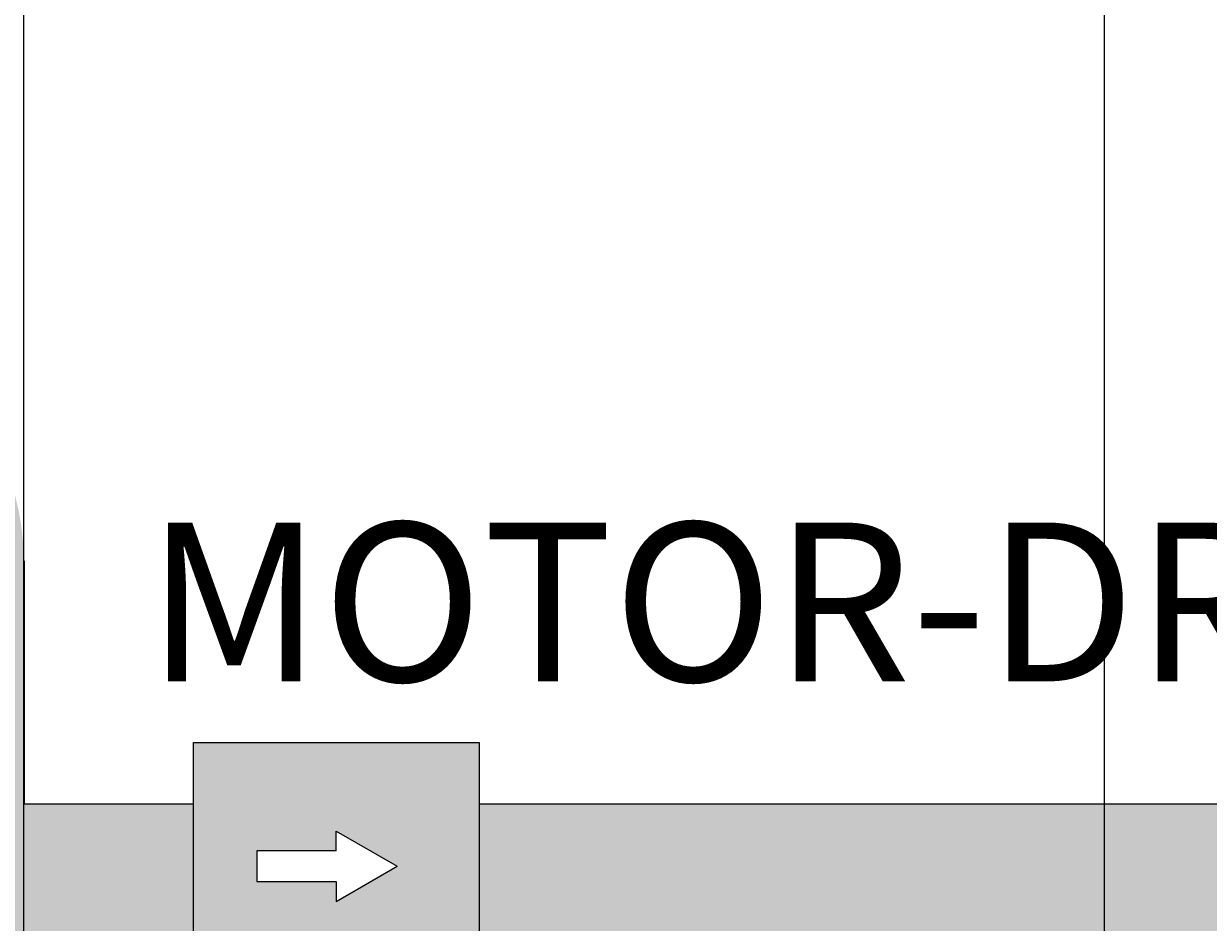
# Model space of a CAD drawing. Units: millimetres. Extents: x -11 to 280, y -4 to 208.
# Tile 41 of 55: x 91 to 121, y 106 to 128. Entities that reach past the tile are written whole.
import ezdxf

# ---------------------------------------------------------------- set-up
doc = ezdxf.new("R2010")
doc.units = ezdxf.units.MM
for name, color, linetype, lineweight in [('M-ANNO-TEXT', 7, 'Continuous', 18), ('M-DIMS', 2, 'Continuous', 18), ('M-HYDR-EQPM', 7, 'Continuous', 35), ('M-HYDR-PRES', 7, 'Continuous', 25), ('M-HYDR-SUCT', 7, 'Continuous', 25), ('M-HYDR-SYMB', 7, 'Continuous', 18), ('M-HYDR-VALV', 7, 'Continuous', 25)]:
    doc.layers.add(name, color=color, linetype=linetype, lineweight=lineweight)
doc.layers.add('M-HYDR-PRES-PATT', color=240, linetype='Continuous', lineweight=13, true_color=0xed1f24)
doc.layers.add('M-HYDR-SUCT-PATT', color=221, linetype='Continuous', lineweight=13, true_color=0xff7fdf)
doc.styles.get("Standard").update_dxf_attribs({"font": 'arial.ttf'})
doc.dimstyles.get("Standard").update_dxf_attribs({"dimtxt": 0.18, "dimasz": 0.18, "dimexe": 0.18, "dimexo": 0.0625, "dimgap": 0.09, "dimtad": 0, "dimtih": 1, "dimtoh": 1, "dimdec": 4, "dimzin": 0, "dimdsep": 46, "dimtxsty": 'Standard', "dimcen": 0.09, "dimadec": 0, "dimazin": 0, "dimtfac": 1, "dimtdec": 4, "dimtofl": 0, "dimtmove": 0, "dimatfit": 3, "dimfxl": 1, "dimtolj": 1, "dimtzin": 0, "dimarcsym": 0})

# ---------------------------------------------------------------- blocks, each defined once
blk = doc.blocks.new('HYDR-FLOW-ARROW')
for p, q in [((2, 1.272), (2, 1.772)), ((2, 1.772), (3.535, 0.886)), ((2, 1.272), (0, 1.272)), ((0, 1.272), (0, 0.5)), ((2, 0), (3.535, 0.886)), ((0, 0.5), (2, 0.5)), ((2, 0.5), (2, 0))]:
    blk.add_line(p, q)
blk = doc.blocks.new('*D5')
at = {"layer": 'Defpoints', "color": 0, "transparency": 16777216}
for p in [(24.759, 192.645), (-10.087, 11.435), (261.686, 11.435)]:
    blk.add_point(p, dxfattribs=at)
at = {"layer": 'M-DIMS', "color": 0, "lineweight": -2, "transparency": 16777216}
for p, q in [((24.696, 192.645), (-10.267, 192.645)), ((-10.087, 192.465), (-10.087, 102.222)), ((-10.087, 11.615), (-10.087, 101.858)), ((261.624, 11.435), (-10.267, 11.435))]:
    blk.add_line(p, q, dxfattribs=at)
at = {"layer": 'M-DIMS', "color": 0, "transparency": 16777216}
for points in [[(-10.117, 192.465), (-10.057, 192.465), (-10.087, 192.645)], [(-10.117, 11.615), (-10.057, 11.615), (-10.087, 11.435)]]:
    blk.add_solid(points, dxfattribs=at)
at = {"layer": 'M-DIMS', "color": 0, "transparency": 16777216, "insert": (-10.087, 102.04), "char_height": 0.18, "attachment_point": 5}
blk.add_mtext('\\A1;181.2', dxfattribs=at)
blk = doc.blocks.new('*D11')
at = {"layer": 'Defpoints', "color": 0, "transparency": 16777216}
for p in [(118.514, 207.495), (91.3, 98.149), (118.514, 96.485)]:
    blk.add_point(p, dxfattribs=at)
at = {"layer": 'M-DIMS', "color": 0, "lineweight": -2, "transparency": 16777216}
for p, q in [((91.3, 98.212), (91.3, 207.675)), ((118.514, 96.547), (118.514, 207.675)), ((91.48, 207.495), (104.442, 207.495)), ((118.334, 207.495), (105.372, 207.495))]:
    blk.add_line(p, q, dxfattribs=at)
at = {"layer": 'M-DIMS', "color": 0, "transparency": 16777216}
for points in [[(91.48, 207.525), (91.48, 207.465), (91.3, 207.495)], [(118.334, 207.525), (118.334, 207.465), (118.514, 207.495)]]:
    blk.add_solid(points, dxfattribs=at)
at = {"layer": 'M-DIMS', "color": 0, "transparency": 16777216, "insert": (104.907, 207.495), "char_height": 0.18, "attachment_point": 5}
blk.add_mtext('\\A1;27.214', dxfattribs=at)
blk = doc.blocks.new('*D12')
at = {"layer": 'Defpoints', "color": 0, "transparency": 16777216}
for p in [(173.804, 207.495), (118.514, 96.485), (173.804, 89.387)]:
    blk.add_point(p, dxfattribs=at)
at = {"layer": 'M-DIMS', "color": 0, "lineweight": -2, "transparency": 16777216}
for p, q in [((118.514, 96.547), (118.514, 207.675)), ((173.804, 89.45), (173.804, 207.675)), ((118.694, 207.495), (145.765, 207.495)), ((173.624, 207.495), (146.553, 207.495))]:
    blk.add_line(p, q, dxfattribs=at)
at = {"layer": 'M-DIMS', "color": 0, "transparency": 16777216}
for points in [[(118.694, 207.525), (118.694, 207.465), (118.514, 207.495)], [(173.624, 207.525), (173.624, 207.465), (173.804, 207.495)]]:
    blk.add_solid(points, dxfattribs=at)
at = {"layer": 'M-DIMS', "color": 0, "transparency": 16777216, "insert": (146.159, 207.495), "char_height": 0.18, "attachment_point": 5}
blk.add_mtext('\\A1;55.29', dxfattribs=at)

msp = doc.modelspace()

# ---------------------------------------------------------------- hatches: boundary and pattern name
at = {"layer": 'M-HYDR-PRES-PATT'}
h = msp.add_hatch(color=256, dxfattribs=at)
h.set_gradient(color1=(237, 31, 36), color2=(237, 31, 36), tint=1)
h.paths.add_polyline_path([(232.2, 133.1228), (228.7, 133.1228), (228.7, 108.8141), (102.7646, 108.8141), (102.7646, 105.3141), (232.2, 105.3141)])
h.paths.add_polyline_path([(128.8433, 105.3141), (125.3433, 105.3141), (125.3433, 91.7099, 1), (128.8433, 91.7099)])
h.paths.add_polyline_path([(229.1617, 78.7098), (196.7745, 78.7098, -0.4142136), (191.7745, 83.7098), (191.7745, 105.3141), (188.2745, 105.3141), (188.2745, 80.2098, 0.4142136), (193.2745, 75.2098), (225.6617, 75.2098), (225.6617, 43.5991), (229.1617, 43.5991)])
h.paths.add_polyline_path([(102.7646, 110.3704), (95.5776, 110.3704), (95.5776, 103.9022), (102.7646, 103.9022)])
h.paths.add_polyline_path([(100.7059, 107.2502), (99.1711, 106.3641), (99.1711, 106.8641), (97.1711, 106.8641), (97.1711, 107.6363), (99.1711, 107.6363), (99.1711, 108.1363)], flags=16)
h.paths.add_polyline_path([(234.6119, 138.4081), (226.5106, 138.4081), (226.5106, 133.1228), (234.6119, 133.1228)])
h.paths.add_polyline_path([(231.1963, 135.7055), (230.2965, 134.1786), (229.4241, 135.7213), (229.9241, 135.7168), (229.9418, 137.7167), (230.7141, 137.7099), (230.6963, 135.71)], flags=16)
at = {"layer": 'M-HYDR-SUCT-PATT'}
h = msp.add_hatch(color=256, dxfattribs=at)
h.set_gradient(color1=(255, 127, 223), color2=(255, 127, 223), tint=1, name='INVCYLINDER')
h.paths.add_polyline_path([(91.3629, 155.4768), (91.3629, 132.4768), (58.3629, 132.4768), (58.3629, 153.9768), (54.8629, 153.9768), (54.8629, 128.9768), (94.8629, 128.9768), (94.8629, 151.9768), (205.5315, 151.9768), (205.5315, 155.4768)])
h.paths.add_polyline_path([(91.3, 114.9452, 1), (78.8273, 114.9452), (78.8273, 108.8141), (42.6453, 108.8141), (42.6453, 153.9768), (39.1453, 153.9768), (39.1453, 105.3141), (78.8273, 105.3141), (78.8273, 98.1491, 1), (91.3, 98.1491), (91.3, 105.3141), (95.5776, 105.3141), (95.5776, 108.8141), (91.3, 108.8141)])
h.paths.add_polyline_path([(228.7, 138.4081), (232.2, 138.4081), (232.2, 144.6609), (228.7, 144.6609)])
h.paths.add_polyline_path([(253.1005, 151.9768, 1), (253.1005, 155.4768), (252.6001, 155.4768), (253.5249, 153.991, -0.1401047), (253.6005, 153.7268, -0.7542249), (252.676, 153.4626), (251.4221, 155.4768), (236.9353, 155.4768), (236.9353, 151.9768)])
h.paths.add_polyline_path([(30.8182, 40.7626), (30.8182, 36.7626), (60.8182, 36.7626), (60.8182, 40.7626)])

# ---------------------------------------------------------------- linework, layer by layer
at = {"layer": 'M-HYDR-EQPM'}
msp.add_lwpolyline([(91.3, 114.9452), (91.3, 108.8141)], dxfattribs=at)
at = {"layer": 'M-HYDR-PRES'}
msp.add_lwpolyline([(228.7, 133.1228), (228.7, 108.8141), (102.7646, 108.8141)], dxfattribs=at)
at = {"layer": 'M-HYDR-SUCT'}
msp.add_lwpolyline([(95.5776, 108.8141), (91.3, 108.8141)], dxfattribs=at)
at = {"layer": 'M-HYDR-VALV'}
msp.add_lwpolyline([(95.5776, 110.3704), (102.7646, 110.3704), (102.7646, 103.9022), (95.5776, 103.9022)], close=True, dxfattribs=at)

# ---------------------------------------------------------------- block references
at = {"layer": 'M-HYDR-SYMB'}
msp.add_blockref('HYDR-FLOW-ARROW', (97.171, 106.364), dxfattribs=at)

# ---------------------------------------------------------------- texts
at = {"layer": 'M-ANNO-TEXT', "insert": (94.3856, 115.9056), "char_height": 4, "attachment_point": 1}
msp.add_mtext_dynamic_manual_height_columns('MOTOR-DRIVEN PUMP', width=63.617875, gutter_width=12.5, heights=[0], dxfattribs=at)

# ---------------------------------------------------------------- dimensions: what is measured, and where the dimension line sits
at = {"layer": 'M-DIMS'}
for base, p1, p2, override, picture, middle in [((118.5137, 207.495), (91.3, 98.1491), (118.5137, 96.4849), {"dimdec": 3, "dimlfac": 1, "dimrnd": 0, "dimzin": 0, "dimdsep": 46, "dimlunit": 2}, '*D11', (104.9068, 207.495)), ((173.8038, 207.495), (118.5137, 96.4849), (173.8038, 89.3873), {"dimdec": 2, "dimlfac": 1, "dimrnd": 0, "dimzin": 0, "dimdsep": 46, "dimlunit": 2}, '*D12', (146.1587, 207.495))]:
    dim = msp.add_linear_dim(base=base, p1=p1, p2=p2, dimstyle='Standard', override=override, dxfattribs=at)
    dim.commit()
    dim.dimension.update_dxf_attribs({"geometry": picture, "text_midpoint": middle})
dim = msp.add_linear_dim(base=(-10.0865, 11.4346), p1=(24.7588, 192.645), p2=(261.6863, 11.4346), angle=90, dimstyle='Standard', override={"dimdec": 1, "dimlfac": 1, "dimrnd": 0, "dimzin": 0, "dimdsep": 46, "dimlunit": 2}, dxfattribs=at)
dim.commit()
dim.dimension.update_dxf_attribs({"geometry": '*D5', "text_midpoint": (-10.0865, 102.0398)})

doc.saveas('drawing.dxf')
